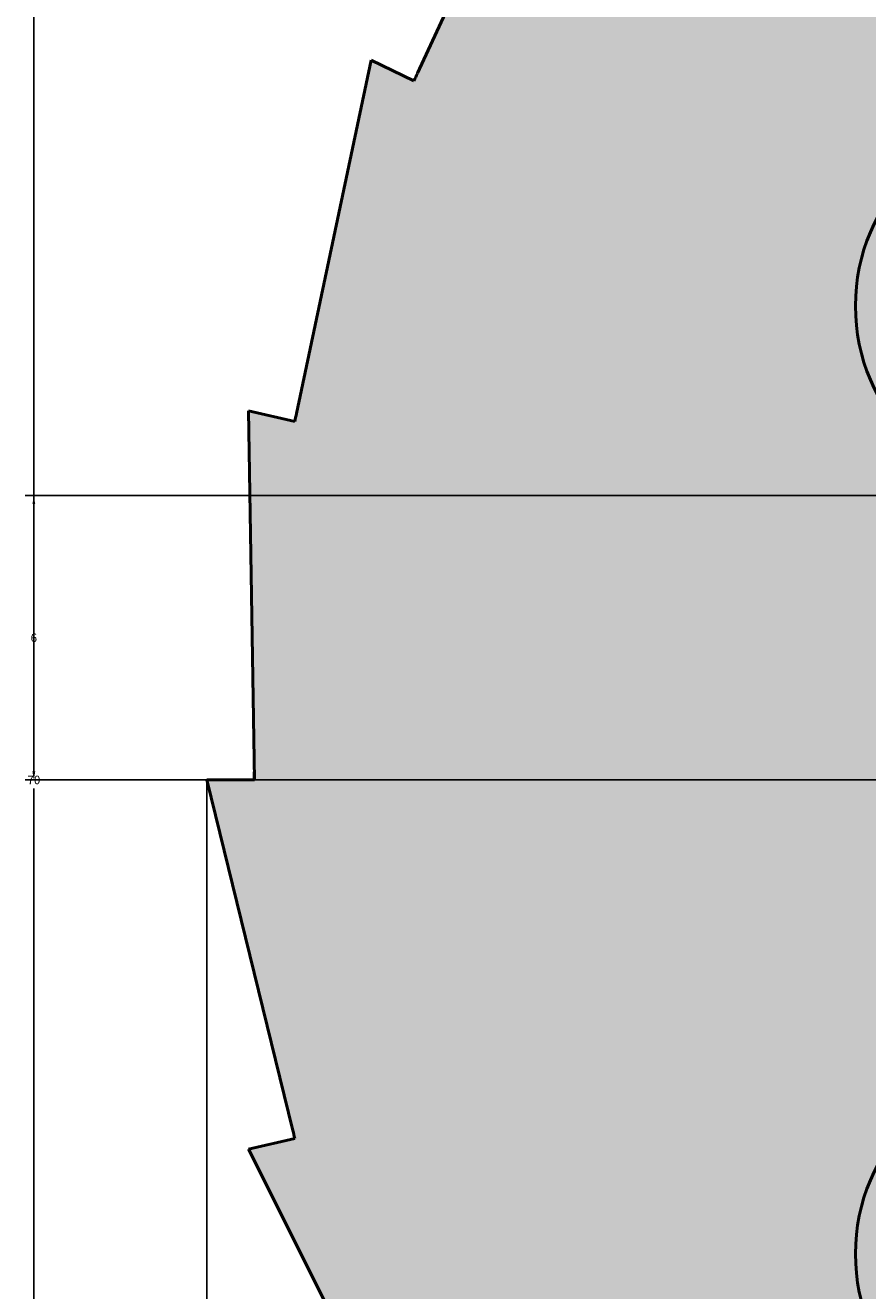
# Model space of a CAD drawing. Units: millimetres. Extents: x 2943.6 to 3032.7, y 1562 to 1639.7.
# Tile 3 of 9: x 2943.6 to 2961.4, y 1590.1 to 1616.8. Entities that reach past the tile are written whole.
import ezdxf

# ---------------------------------------------------------------- set-up
doc = ezdxf.new("R2010")
doc.units = ezdxf.units.MM
doc.layers.add('M-DIMS', color=2, linetype='Continuous', lineweight=18)
doc.layers.add('M-OUTL', color=7, linetype='Continuous', lineweight=50)
doc.layers.add('M-HATC', color=7, linetype='Continuous', lineweight=18, true_color=0xffffff)
doc.styles.get("Standard").update_dxf_attribs({"font": 'arial.ttf'})
doc.dimstyles.get("Standard").update_dxf_attribs({"dimtxt": 0.18, "dimasz": 0.18, "dimexe": 0.18, "dimexo": 0.0625, "dimgap": 0.09, "dimtad": 0, "dimtih": 1, "dimtoh": 1, "dimdec": 4, "dimzin": 0, "dimdsep": 46, "dimtxsty": 'Standard', "dimcen": 0.09, "dimadec": 0, "dimazin": 0, "dimtfac": 1, "dimtdec": 4, "dimtofl": 0, "dimtmove": 0, "dimatfit": 3, "dimfxl": 1, "dimtolj": 1, "dimtzin": 0, "dimarcsym": 0})

# ---------------------------------------------------------------- blocks, each defined once
blk = doc.blocks.new('*U1')
blk.add_circle((0, 0), 4)
blk = doc.blocks.new('*U2')
at = {"layer": 'M-OUTL', "color": 0, "linetype": 'ByBlock', "lineweight": -2, "transparency": 16777216}
for p, rotation in [((2965.149, 1610.848), 59.99999999999999), ((2965.149, 1590.848), 120)]:
    blk.add_blockref('*U1', p, dxfattribs=dict(at, rotation=rotation))
blk = doc.blocks.new('*D3')
at = {"layer": 'Defpoints', "color": 0, "transparency": 16777216}
for p in [(2947.469, 1600.848), (3017.469, 1600.848), (3017.469, 1562.198)]:
    blk.add_point(p, dxfattribs=at)
at = {"layer": 'M-DIMS', "color": 0, "lineweight": -2, "transparency": 16777216}
for p, q in [((2947.469, 1600.786), (2947.469, 1562.018)), ((3017.469, 1600.786), (3017.469, 1562.018)), ((2947.649, 1562.198), (2982.251, 1562.198)), ((3017.289, 1562.198), (2982.687, 1562.198))]:
    blk.add_line(p, q, dxfattribs=at)
at = {"layer": 'M-DIMS', "color": 0, "transparency": 16777216}
for points in [[(2947.649, 1562.228), (2947.649, 1562.168), (2947.469, 1562.198)], [(3017.289, 1562.228), (3017.289, 1562.168), (3017.469, 1562.198)]]:
    blk.add_solid(points, dxfattribs=at)
at = {"layer": 'M-DIMS', "color": 0, "transparency": 16777216, "insert": (2982.469, 1562.198), "char_height": 0.18, "attachment_point": 5}
blk.add_mtext('\\A1;70', dxfattribs=at)
blk = doc.blocks.new('*D4')
at = {"layer": 'Defpoints', "color": 0, "transparency": 16777216}
for p in [(2943.819, 1635.848), (2982.469, 1635.848), (2982.469, 1565.848)]:
    blk.add_point(p, dxfattribs=at)
at = {"layer": 'M-DIMS', "color": 0, "lineweight": -2, "transparency": 16777216}
for p, q in [((2982.407, 1635.848), (2943.639, 1635.848)), ((2943.819, 1635.668), (2943.819, 1601.03)), ((2943.819, 1566.028), (2943.819, 1600.666)), ((2982.407, 1565.848), (2943.639, 1565.848))]:
    blk.add_line(p, q, dxfattribs=at)
at = {"layer": 'M-DIMS', "color": 0, "transparency": 16777216}
for points in [[(2943.789, 1635.668), (2943.849, 1635.668), (2943.819, 1635.848)], [(2943.789, 1566.028), (2943.849, 1566.028), (2943.819, 1565.848)]]:
    blk.add_solid(points, dxfattribs=at)
at = {"layer": 'M-DIMS', "color": 0, "transparency": 16777216, "insert": (2943.819, 1600.848), "char_height": 0.18, "attachment_point": 5}
blk.add_mtext('\\A1;70', dxfattribs=at)
blk = doc.blocks.new('*D9')
at = {"layer": 'Defpoints', "color": 0, "transparency": 16777216}
for p in [(2943.819, 1606.848), (2981.469, 1606.848), (2982.469, 1600.848)]:
    blk.add_point(p, dxfattribs=at)
at = {"layer": 'M-DIMS', "color": 0, "lineweight": -2, "transparency": 16777216}
for p, q in [((2981.407, 1606.848), (2943.639, 1606.848)), ((2943.819, 1606.668), (2943.819, 1604.03)), ((2943.819, 1601.028), (2943.819, 1603.666)), ((2982.407, 1600.848), (2943.639, 1600.848))]:
    blk.add_line(p, q, dxfattribs=at)
at = {"layer": 'M-DIMS', "color": 0, "transparency": 16777216}
for points in [[(2943.789, 1606.668), (2943.849, 1606.668), (2943.819, 1606.848)], [(2943.789, 1601.028), (2943.849, 1601.028), (2943.819, 1600.848)]]:
    blk.add_solid(points, dxfattribs=at)
at = {"layer": 'M-DIMS', "color": 0, "transparency": 16777216, "insert": (2943.819, 1603.848), "char_height": 0.18, "attachment_point": 5}
blk.add_mtext('\\A1;6', dxfattribs=at)

msp = doc.modelspace()

# ---------------------------------------------------------------- hatches: boundary and pattern name
at = {"layer": 'M-HATC'}
h = msp.add_hatch(color=256, dxfattribs=at)
h.set_gradient(color1=(0, 0, 255), color2=(255, 255, 0), tint=1, name='INVCURVED')
h.paths.add_polyline_path([(2949.361, 1608.583, 0.001279), (2949.322, 1608.414), (2948.347, 1608.637), (2948.473, 1600.848), (2947.469, 1600.848), (2949.283, 1593.452, 0.001279), (2949.322, 1593.283), (2948.347, 1593.06), (2951.761, 1586.253, 0.001279), (2951.836, 1586.096), (2950.935, 1585.662), (2955.779, 1579.786, 0.001279), (2955.887, 1579.65), (2955.105, 1579.026), (2961.135, 1574.375, 0.001279), (2961.271, 1574.266), (2960.647, 1573.484), (2967.561, 1570.291, 0.001279), (2967.717, 1570.215), (2967.283, 1569.314), (2974.734, 1567.74, 0.001279), (2974.904, 1567.701), (2974.681, 1566.726), (2982.295, 1566.849, 0.001279), (2982.469, 1566.848), (2982.469, 1565.848), (2989.865, 1567.662, 0.001279), (2990.035, 1567.701), (2990.258, 1566.726), (2997.064, 1570.14, 0.001279), (2997.221, 1570.215), (2997.655, 1569.314), (3003.532, 1574.158, 0.001279), (3003.668, 1574.266), (3004.291, 1573.484), (3008.943, 1579.514, 0.001279), (3009.052, 1579.65), (3009.833, 1579.026), (3013.026, 1585.94, 0.001279), (3013.102, 1586.096), (3014.003, 1585.662), (3015.578, 1593.113, 0.001279), (3015.617, 1593.283), (3016.592, 1593.06), (3016.469, 1600.674, 0.001279), (3016.469, 1600.848), (3017.469, 1600.848), (3015.655, 1608.244, 0.001279), (3015.617, 1608.414), (3016.592, 1608.637), (3013.177, 1615.443, 0.001279), (3013.102, 1615.6), (3014.003, 1616.034), (3009.16, 1621.911, 0.001279), (3009.052, 1622.047), (3009.833, 1622.67), (3003.804, 1627.322, 0.001279), (3003.668, 1627.431), (3004.291, 1628.212), (2997.378, 1631.405, 0.001279), (2997.221, 1631.481), (2997.655, 1632.382), (2990.204, 1633.957, 0.001279), (2990.035, 1633.996), (2990.258, 1634.971), (2982.469, 1634.845), (2982.469, 1635.848), (2975.073, 1634.034, 0.001279), (2974.904, 1633.996), (2974.681, 1634.971), (2967.874, 1631.556, 0.001279), (2967.717, 1631.481), (2967.283, 1632.382), (2961.407, 1627.539, 0.001279), (2961.271, 1627.431), (2960.647, 1628.212), (2955.996, 1622.183, 0.001279), (2955.887, 1622.047), (2955.105, 1622.67), (2951.912, 1615.757, 0.001279), (2951.836, 1615.6), (2950.935, 1616.034)])
h.paths.add_polyline_path([(2969.149, 1610.848, -1), (2961.149, 1610.848, -1)], flags=16)
h.paths.add_polyline_path([(2969.149, 1590.848, -1), (2961.149, 1590.848, -1)], flags=16)
h.paths.add_polyline_path([(2992.469, 1600.848, -1), (2972.469, 1600.848, -1)], flags=16)
h.paths.add_polyline_path([(2978.469, 1620.848, -1), (2986.469, 1620.848, -1)], flags=16)
h.paths.add_polyline_path([(2981.469, 1605.236), (2981.469, 1606.848), (2983.469, 1606.848), (2983.469, 1605.236, -8.887482)], flags=0)
h.paths.add_polyline_path([(2986.469, 1580.848, -1), (2978.469, 1580.848, -1)], flags=16)
h.paths.add_polyline_path([(3003.79, 1610.848, -1), (2995.79, 1610.848, -1)], flags=16)
h.paths.add_polyline_path([(3003.79, 1590.848, -1), (2995.79, 1590.848, -1)], flags=16)
h = msp.add_hatch(color=256, dxfattribs=at)
h.paths.add_polyline_path([(2978.469, 1620.848, 1), (2986.469, 1620.848, 1)])
h.paths.add_polyline_path([(2995.79, 1610.848, 1), (3003.79, 1610.848, 1)])
h.paths.add_polyline_path([(3003.79, 1590.848, 1), (2995.79, 1590.848, 1)])
h.paths.add_polyline_path([(2986.469, 1580.848, 1), (2978.469, 1580.848, 1)])
h.paths.add_polyline_path([(2969.149, 1590.848, 1), (2961.149, 1590.848, 1)])
h.paths.add_polyline_path([(2961.149, 1610.848, 1), (2969.149, 1610.848, 1)])

# ---------------------------------------------------------------- linework, layer by layer
at = {"layer": 'M-OUTL'}
for p, q in [((2951.912, 1615.757), (2955.105, 1622.67)), ((2949.361, 1608.583), (2950.935, 1616.034)), ((2951.836, 1615.6), (2950.935, 1616.034)), ((2949.322, 1608.414), (2948.347, 1608.637)), ((2948.473, 1600.848), (2948.347, 1608.637)), ((2947.469, 1600.848), (2948.473, 1600.848)), ((2948.469, 1600.848), (2947.469, 1600.848)), ((2949.283, 1593.452), (2947.469, 1600.848)), ((2949.322, 1593.283), (2948.347, 1593.06)), ((2951.761, 1586.253), (2948.347, 1593.06))]:
    msp.add_line(p, q, dxfattribs=at)
for start, end in [(153.9926, 154.2857), (166.8498, 167.1429), (179.7069, 180), (192.564, 192.8571)]:
    msp.add_arc((2982.469, 1600.848), 34, start, end, dxfattribs=at)

# ---------------------------------------------------------------- block references
msp.add_blockref('*U2', (0, 0), dxfattribs=at)

# ---------------------------------------------------------------- dimensions: what is measured, and where the dimension line sits
at = {"layer": 'M-DIMS'}
for base, p1, p2, picture, middle in [((2943.819, 1635.848), (2982.469, 1565.848), (2982.469, 1635.848), '*D4', (2943.819, 1600.848)), ((2943.819, 1606.848), (2982.469, 1600.848), (2981.469, 1606.848), '*D9', (2943.819, 1603.848))]:
    dim = msp.add_linear_dim(base=base, p1=p1, p2=p2, angle=90, dimstyle='Standard', override={"dimdec": 0, "dimlfac": 1, "dimrnd": 0, "dimzin": 0, "dimdsep": 46, "dimlunit": 2}, dxfattribs=at)
    dim.commit()
    dim.dimension.update_dxf_attribs({"geometry": picture, "text_midpoint": middle})
dim = msp.add_linear_dim(base=(3017.469, 1562.198), p1=(2947.469, 1600.848), p2=(3017.469, 1600.848), dimstyle='Standard', override={"dimdec": 0, "dimlfac": 1, "dimrnd": 0, "dimzin": 0, "dimdsep": 46, "dimlunit": 2}, dxfattribs=at)
dim.commit()
dim.dimension.update_dxf_attribs({"geometry": '*D3', "text_midpoint": (2982.469, 1562.198)})

doc.saveas('drawing.dxf')
